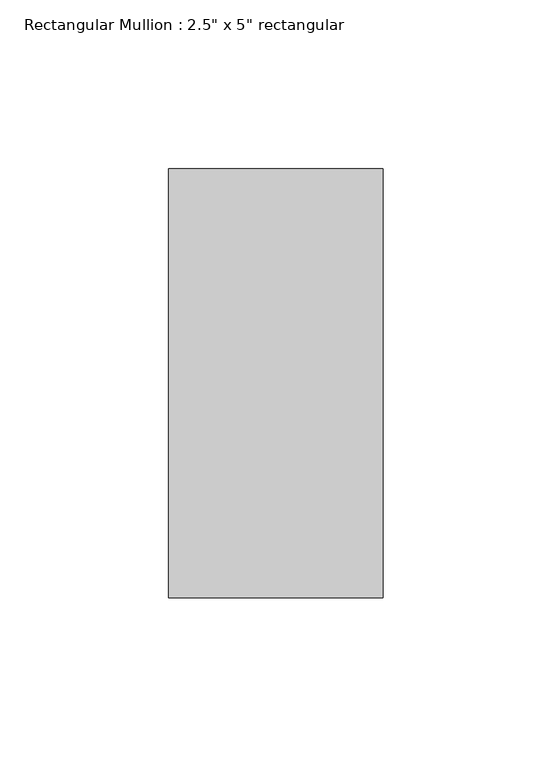
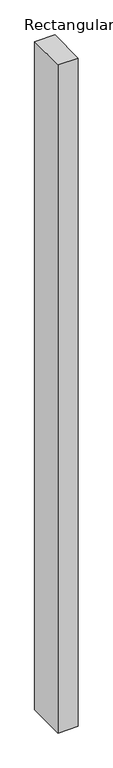
"""IFC4 building model written with IfcOpenShell, lengths in millimetres: member geometry."""

from ifc_helpers import new_model, si_unit, frame, origin, place, context, project, spatial, polyline, outline, extrude, source, transform, mapped, element, save


def member_3a21dca5(model_context):
    return source(origin(), model_context, "Body", "SweptSolid", [
        extrude(outline(polyline([(0.0, 63.5), (0.0, -63.5), (-63.5, -63.5), (-63.5, 63.5), (0.0, 63.5)])), frame((0.0, 0.0, -2227.7840877), z_axis=(0.0, 0.0, 1.0), x_axis=(1.0, 0.0, 0.0)), (0.0, 0.0, 1.0), 2227.7840877),
    ])


if __name__ == "__main__":
    model = new_model("IFC4")
    model_context = context("Model", 3, world=origin())
    ifc_project = project(units=[si_unit("LENGTHUNIT", "METRE", prefix="MILLI")], contexts=[model_context])
    site = spatial("IfcSite", under=ifc_project)
    building = spatial("IfcBuilding", under=site)
    placement = place(None, origin())
    member_shape = member_3a21dca5(model_context)
    element("IfcMember", 1, ObjectType="Rectangular Mullion : 2.5\" x 5\" rectangular", at=placement, inside=building, context=model_context, shape_type="MappedRepresentation", body=[
        mapped(member_shape, transform((0.0, 0.0, 0.0), x_axis=(1.0, 0.0, 0.0), y_axis=(0.0, 1.0, 0.0), z_axis=(0.0, 0.0, 1.0))),
    ])
    save(model, "model.ifc")

# Revit data of these elements
# Type "Rectangular Mullion : 2.5\" x 5\" rectangular"
#   built-in parameter 1007304 = 0.416667 (stored number, unit not read)
#   built-in parameter 1007301 = 0.104167 (stored number, unit not read)
#   built-in parameter 1007300 = 0.104167 (stored number, unit not read)
# Element 1 (IfcMember, "Rectangular Mullion : 2.5\" x 5\" rectangular")
#   Materials on its faces: "Aluminum"
# Materials
#   "Aluminum": class "Metal", colour RGB 247 247 247, transparency 0, Description = "Aluminum 6061", Cost = 0
